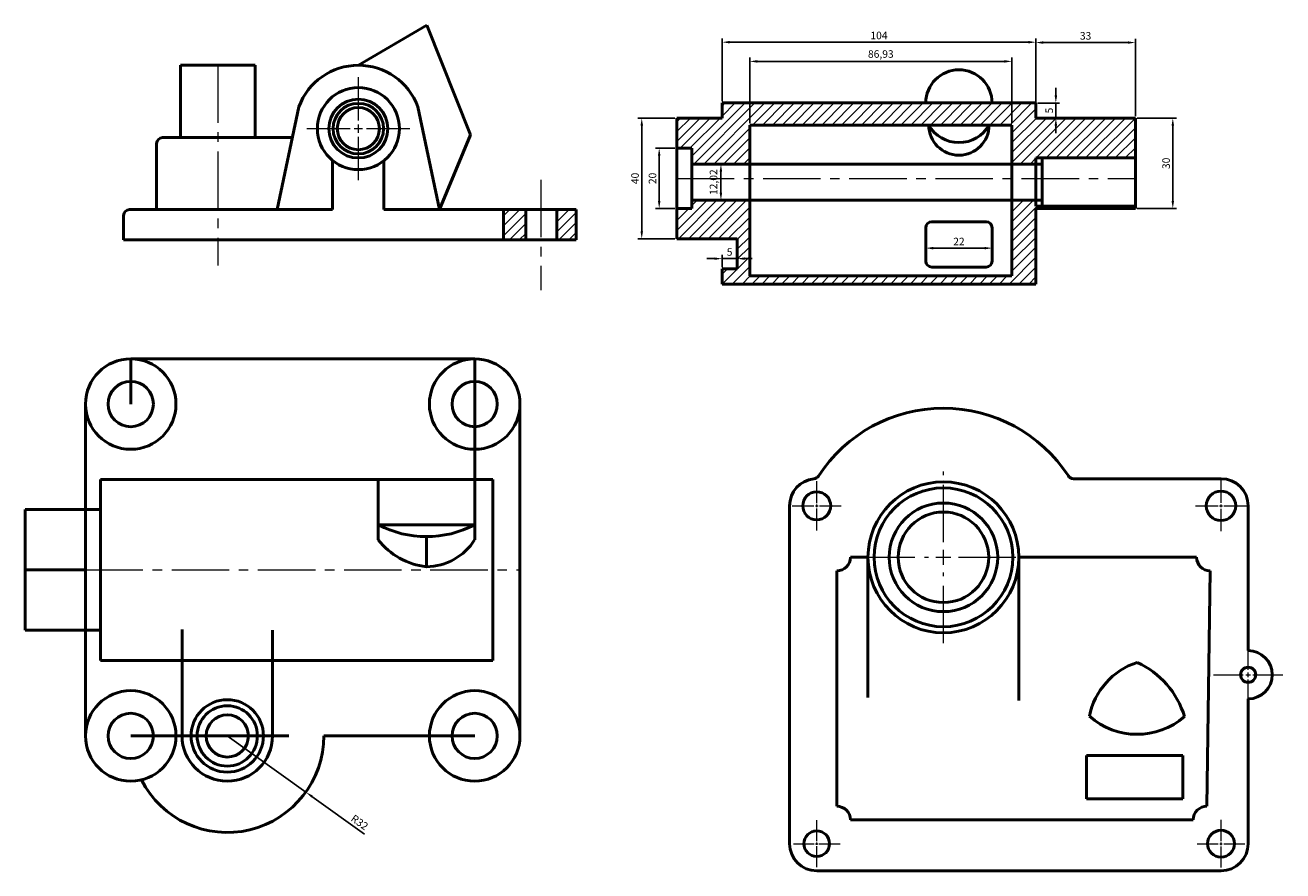
# Model space of a CAD drawing. Units: millimetres. Extents: x 1096 to 1848, y 1781 to 2075.
# Tile 1 of 2: x 1096 to 1513, y 1795 to 2075. Entities that reach past the tile are written whole.
import ezdxf

# ---------------------------------------------------------------- set-up
doc = ezdxf.new("R2010")
doc.units = ezdxf.units.MM
doc.linetypes.add('CENTER2', pattern=[28.575, 19.05, -3.175, 3.175, -3.175])
for name, color, linetype, lineweight in [('M-CNTR', 1, 'CENTER2', 18), ('M-DIMS', 2, 'Continuous', 25), ('M-HATC', 8, 'Continuous', 18), ('M-OUTL', 7, 'Continuous', 50)]:
    doc.layers.add(name, color=color, linetype=linetype, lineweight=lineweight)
doc.styles.get("Standard").update_dxf_attribs({"font": 'arial.ttf'})
doc.dimstyles.new('ISO-25', dxfattribs={"dimtxt": 2.5, "dimasz": 2.5, "dimexe": 1.25, "dimexo": 0.625, "dimtad": 1, "dimtxsty": 'Standard', "dimcen": 2.5, "dimadec": 0, "dimazin": 0, "dimtfac": 1, "dimtmove": 0, "dimatfit": 3, "dimfxl": 1, "dimarcsym": 0})

# ---------------------------------------------------------------- blocks, each defined once
blk = doc.blocks.new('*U1')
at = {"layer": 'M-CNTR', "color": 0, "transparency": 16777216}
for p, q in [((0, 2.72), (0, 17.09)), ((-17.09, 0), (-2.72, 0)), ((2.72, 0), (17.09, 0)), ((0, -17.09), (0, -2.72))]:
    blk.add_line(p, q, dxfattribs=at)
at = {"layer": 'M-CNTR', "color": 0, "linetype": 'Continuous', "transparency": 16777216}
for p, q in [((-1.36, 0), (1.36, 0)), ((0, -1.36), (0, 1.36))]:
    blk.add_line(p, q, dxfattribs=at)
blk = doc.blocks.new('*D2')
at = {"layer": 'Defpoints', "color": 0, "transparency": 16777216}
for p in [(1431.45, 2069.78), (1327.45, 2049.62), (1431.45, 2049.62)]:
    blk.add_point(p, dxfattribs=at)
at = {"layer": 'M-DIMS', "color": 0, "lineweight": -2, "transparency": 16777216}
for p, q in [((1327.45, 2050.25), (1327.45, 2071.03)), ((1329.95, 2069.78), (1428.95, 2069.78)), ((1431.45, 2050.25), (1431.45, 2071.03))]:
    blk.add_line(p, q, dxfattribs=at)
at = {"layer": 'M-DIMS', "color": 0, "transparency": 16777216}
for points in [[(1329.95, 2070.2), (1329.95, 2069.37), (1327.45, 2069.78)], [(1428.95, 2070.2), (1428.95, 2069.37), (1431.45, 2069.78)]]:
    blk.add_solid(points, dxfattribs=at)
at = {"layer": 'M-DIMS', "color": 0, "transparency": 16777216, "insert": (1379.45, 2071.68), "char_height": 2.5, "attachment_point": 5}
blk.add_mtext('104', dxfattribs=at)
blk = doc.blocks.new('*D3')
at = {"layer": 'Defpoints', "color": 0, "transparency": 16777216}
for p in [(1423.53, 2063.42), (1336.6, 2042.31), (1423.53, 2042.31)]:
    blk.add_point(p, dxfattribs=at)
at = {"layer": 'M-DIMS', "color": 0, "lineweight": -2, "transparency": 16777216}
for p, q in [((1336.6, 2042.94), (1336.6, 2064.67)), ((1423.53, 2042.94), (1423.53, 2064.67)), ((1339.1, 2063.42), (1421.03, 2063.42))]:
    blk.add_line(p, q, dxfattribs=at)
at = {"layer": 'M-DIMS', "color": 0, "transparency": 16777216}
for points in [[(1339.1, 2063.83), (1339.1, 2063), (1336.6, 2063.42)], [(1421.03, 2063.83), (1421.03, 2063), (1423.53, 2063.42)]]:
    blk.add_solid(points, dxfattribs=at)
at = {"layer": 'M-DIMS', "color": 0, "transparency": 16777216, "insert": (1380.07, 2065.54), "char_height": 2.5, "attachment_point": 5}
blk.add_mtext('86,93', dxfattribs=at)
blk = doc.blocks.new('*D4')
at = {"layer": 'Defpoints', "color": 0, "transparency": 16777216}
for p in [(1464.45, 2044.62), (1464.45, 2014.62), (1476.86, 2014.62)]:
    blk.add_point(p, dxfattribs=at)
at = {"layer": 'M-DIMS', "color": 0, "lineweight": -2, "transparency": 16777216}
for p, q in [((1465.08, 2044.62), (1478.11, 2044.62)), ((1476.86, 2042.12), (1476.86, 2017.12)), ((1465.08, 2014.62), (1478.11, 2014.62))]:
    blk.add_line(p, q, dxfattribs=at)
at = {"layer": 'M-DIMS', "color": 0, "transparency": 16777216}
for points in [[(1476.44, 2042.12), (1477.27, 2042.12), (1476.86, 2044.62)], [(1476.44, 2017.12), (1477.27, 2017.12), (1476.86, 2014.62)]]:
    blk.add_solid(points, dxfattribs=at)
at = {"layer": 'M-DIMS', "color": 0, "transparency": 16777216, "insert": (1474.96, 2029.62), "char_height": 2.5, "attachment_point": 5, "rotation": 90}
blk.add_mtext('30', dxfattribs=at)
blk = doc.blocks.new('*D5')
at = {"layer": 'Defpoints', "color": 0, "transparency": 16777216}
for p in [(1394.96, 2002.73), (1416.96, 2002.73), (1416.96, 2001.51)]:
    blk.add_point(p, dxfattribs=at)
at = {"layer": 'M-DIMS', "color": 0, "lineweight": -2, "transparency": 16777216}
for p, q in [((1394.96, 2002.11), (1394.96, 2000.26)), ((1397.46, 2001.51), (1414.46, 2001.51)), ((1416.96, 2002.11), (1416.96, 2000.26))]:
    blk.add_line(p, q, dxfattribs=at)
at = {"layer": 'M-DIMS', "color": 0, "transparency": 16777216}
for points in [[(1397.46, 2001.92), (1397.46, 2001.09), (1394.96, 2001.51)], [(1414.46, 2001.92), (1414.46, 2001.09), (1416.96, 2001.51)]]:
    blk.add_solid(points, dxfattribs=at)
at = {"layer": 'M-DIMS', "color": 0, "transparency": 16777216, "insert": (1405.96, 2003.39), "char_height": 2.5, "attachment_point": 5}
blk.add_mtext('22', dxfattribs=at)
blk = doc.blocks.new('*D6')
at = {"layer": 'Defpoints', "color": 0, "transparency": 16777216}
for p in [(1332.45, 1998.03), (1327.45, 1994.62), (1332.45, 1994.62)]:
    blk.add_point(p, dxfattribs=at)
at = {"layer": 'M-DIMS', "color": 0, "lineweight": -2, "transparency": 16777216}
for p, q in [((1324.95, 1998.03), (1322.45, 1998.03)), ((1327.45, 1995.25), (1327.45, 1999.28)), ((1327.45, 1998.03), (1332.45, 1998.03)), ((1332.45, 1995.25), (1332.45, 1999.28)), ((1334.95, 1998.03), (1337.45, 1998.03))]:
    blk.add_line(p, q, dxfattribs=at)
at = {"layer": 'M-DIMS', "color": 0, "transparency": 16777216}
for points in [[(1324.95, 1998.44), (1324.95, 1997.61), (1327.45, 1998.03)], [(1334.95, 1998.44), (1334.95, 1997.61), (1332.45, 1998.03)]]:
    blk.add_solid(points, dxfattribs=at)
at = {"layer": 'M-DIMS', "color": 0, "transparency": 16777216, "insert": (1329.95, 1999.92), "char_height": 2.5, "attachment_point": 5}
blk.add_mtext('5', dxfattribs=at)
blk = doc.blocks.new('*D7')
at = {"layer": 'Defpoints', "color": 0, "transparency": 16777216}
for p in [(1312.45, 2044.62), (1300.83, 2004.62), (1312.45, 2004.62)]:
    blk.add_point(p, dxfattribs=at)
at = {"layer": 'M-DIMS', "color": 0, "lineweight": -2, "transparency": 16777216}
for p, q in [((1311.83, 2044.62), (1299.58, 2044.62)), ((1300.83, 2042.12), (1300.83, 2007.12)), ((1311.83, 2004.62), (1299.58, 2004.62))]:
    blk.add_line(p, q, dxfattribs=at)
at = {"layer": 'M-DIMS', "color": 0, "transparency": 16777216}
for points in [[(1300.41, 2042.12), (1301.25, 2042.12), (1300.83, 2044.62)], [(1300.41, 2007.12), (1301.25, 2007.12), (1300.83, 2004.62)]]:
    blk.add_solid(points, dxfattribs=at)
at = {"layer": 'M-DIMS', "color": 0, "transparency": 16777216, "insert": (1298.93, 2024.62), "char_height": 2.5, "attachment_point": 5, "rotation": 90}
blk.add_mtext('40', dxfattribs=at)
blk = doc.blocks.new('*D8')
at = {"layer": 'Defpoints', "color": 0, "transparency": 16777216}
for p in [(1312.45, 2034.62), (1306.61, 2014.62), (1312.45, 2014.62)]:
    blk.add_point(p, dxfattribs=at)
at = {"layer": 'M-DIMS', "color": 0, "lineweight": -2, "transparency": 16777216}
for p, q in [((1311.83, 2034.62), (1305.36, 2034.62)), ((1306.61, 2032.12), (1306.61, 2017.12)), ((1311.83, 2014.62), (1305.36, 2014.62))]:
    blk.add_line(p, q, dxfattribs=at)
at = {"layer": 'M-DIMS', "color": 0, "transparency": 16777216}
for points in [[(1306.19, 2032.12), (1307.03, 2032.12), (1306.61, 2034.62)], [(1306.19, 2017.12), (1307.03, 2017.12), (1306.61, 2014.62)]]:
    blk.add_solid(points, dxfattribs=at)
at = {"layer": 'M-DIMS', "color": 0, "transparency": 16777216, "insert": (1304.71, 2024.62), "char_height": 2.5, "attachment_point": 5, "rotation": 90}
blk.add_mtext('20', dxfattribs=at)
blk = doc.blocks.new('*D9')
at = {"layer": 'Defpoints', "color": 0, "transparency": 16777216}
for p in [(1317.45, 2029.39), (1317.45, 2017.37), (1327.07, 2017.37)]:
    blk.add_point(p, dxfattribs=at)
at = {"layer": 'M-DIMS', "color": 0, "lineweight": -2, "transparency": 16777216}
for p, q in [((1318.08, 2029.39), (1328.32, 2029.39)), ((1327.07, 2026.89), (1327.07, 2019.87)), ((1318.08, 2017.37), (1328.32, 2017.37))]:
    blk.add_line(p, q, dxfattribs=at)
at = {"layer": 'M-DIMS', "color": 0, "transparency": 16777216}
for points in [[(1326.65, 2026.89), (1327.48, 2026.89), (1327.07, 2029.39)], [(1326.65, 2019.87), (1327.48, 2019.87), (1327.07, 2017.37)]]:
    blk.add_solid(points, dxfattribs=at)
at = {"layer": 'M-DIMS', "color": 0, "transparency": 16777216, "insert": (1324.94, 2023.38), "char_height": 2.5, "attachment_point": 5, "rotation": 90}
blk.add_mtext('12,02', dxfattribs=at)
blk = doc.blocks.new('*D10')
at = {"layer": 'Defpoints', "color": 0, "transparency": 16777216}
for p in [(1464.45, 2069.66), (1431.45, 2044.62), (1464.45, 2044.62)]:
    blk.add_point(p, dxfattribs=at)
at = {"layer": 'M-DIMS', "color": 0, "lineweight": -2, "transparency": 16777216}
for p, q in [((1431.45, 2045.25), (1431.45, 2070.91)), ((1433.95, 2069.66), (1461.95, 2069.66)), ((1464.45, 2045.25), (1464.45, 2070.91))]:
    blk.add_line(p, q, dxfattribs=at)
at = {"layer": 'M-DIMS', "color": 0, "transparency": 16777216}
for points in [[(1433.95, 2070.08), (1433.95, 2069.24), (1431.45, 2069.66)], [(1461.95, 2070.08), (1461.95, 2069.24), (1464.45, 2069.66)]]:
    blk.add_solid(points, dxfattribs=at)
at = {"layer": 'M-DIMS', "color": 0, "transparency": 16777216, "insert": (1447.95, 2071.56), "char_height": 2.5, "attachment_point": 5}
blk.add_mtext('33', dxfattribs=at)
blk = doc.blocks.new('*D11')
at = {"layer": 'Defpoints', "color": 0, "transparency": 16777216}
for p in [(1431.45, 2049.62), (1431.45, 2044.62), (1438.09, 2044.62)]:
    blk.add_point(p, dxfattribs=at)
at = {"layer": 'M-DIMS', "color": 0, "lineweight": -2, "transparency": 16777216}
for p, q in [((1438.09, 2052.12), (1438.09, 2054.62)), ((1432.08, 2049.62), (1439.34, 2049.62)), ((1438.09, 2049.62), (1438.09, 2044.62)), ((1432.08, 2044.62), (1439.34, 2044.62)), ((1438.09, 2042.12), (1438.09, 2039.62))]:
    blk.add_line(p, q, dxfattribs=at)
at = {"layer": 'M-DIMS', "color": 0, "transparency": 16777216}
for points in [[(1437.68, 2052.12), (1438.51, 2052.12), (1438.09, 2049.62)], [(1437.68, 2042.12), (1438.51, 2042.12), (1438.09, 2044.62)]]:
    blk.add_solid(points, dxfattribs=at)
at = {"layer": 'M-DIMS', "color": 0, "transparency": 16777216, "insert": (1436.2, 2047.12), "char_height": 2.5, "attachment_point": 5, "rotation": 90}
blk.add_mtext('5', dxfattribs=at)
blk = doc.blocks.new('*D12')
at = {"layer": 'Defpoints', "color": 0, "transparency": 16777216}
for p in [(1163.45, 1839.83), (1189.47, 1821.21)]:
    blk.add_point(p, dxfattribs=at)
at = {"layer": 'M-DIMS', "color": 0, "lineweight": -2, "transparency": 16777216}
for p, q in [((1163.45, 1839.83), (1189.47, 1821.21)), ((1208.96, 1807.28), (1191.51, 1819.76))]:
    blk.add_line(p, q, dxfattribs=at)
at = {"layer": 'M-DIMS', "color": 0, "transparency": 16777216}
blk.add_solid([(1191.75, 1820.1), (1191.27, 1819.42), (1189.47, 1821.21)], dxfattribs=at)
at = {"layer": 'M-DIMS', "color": 0, "transparency": 16777216, "insert": (1207.13, 1810.92), "char_height": 2.5, "attachment_point": 5, "rotation": 324.4294}
blk.add_mtext('R32', dxfattribs=at)
blk = doc.blocks.new('*U29')
at = {"layer": 'M-CNTR', "color": 0, "transparency": 16777216}
for p, q in [((0, 1.6), (0, 11.5)), ((-11.5, 0), (-1.6, 0)), ((1.6, 0), (11.5, 0)), ((0, -11.5), (0, -1.6))]:
    blk.add_line(p, q, dxfattribs=at)
at = {"layer": 'M-CNTR', "color": 0, "linetype": 'Continuous', "transparency": 16777216}
for p, q in [((-0.8, 0), (0.8, 0)), ((0, -0.8), (0, 0.8))]:
    blk.add_line(p, q, dxfattribs=at)
blk = doc.blocks.new('*U30')
at = {"layer": 'M-CNTR', "color": 0, "transparency": 16777216}
for p, q in [((0, 0.98), (0, 8.4)), ((-8.4, 0), (-0.98, 0)), ((0.98, 0), (8.4, 0)), ((0, -8.4), (0, -0.98))]:
    blk.add_line(p, q, dxfattribs=at)
at = {"layer": 'M-CNTR', "color": 0, "linetype": 'Continuous', "transparency": 16777216}
for p, q in [((-0.49, 0), (0.49, 0)), ((0, -0.49), (0, 0.49))]:
    blk.add_line(p, q, dxfattribs=at)
blk = doc.blocks.new('*U31')
at = {"layer": 'M-CNTR', "color": 0, "transparency": 16777216}
for p, q in [((0, 0.93), (0, 8.14)), ((-8.14, 0), (-0.93, 0)), ((0.93, 0), (8.14, 0)), ((0, -8.14), (0, -0.93))]:
    blk.add_line(p, q, dxfattribs=at)
at = {"layer": 'M-CNTR', "color": 0, "linetype": 'Continuous', "transparency": 16777216}
for p, q in [((-0.46, 0), (0.46, 0)), ((0, -0.46), (0, 0.46))]:
    blk.add_line(p, q, dxfattribs=at)
blk = doc.blocks.new('*U32')
at = {"layer": 'M-CNTR', "color": 0, "transparency": 16777216}
for p, q in [((0, 0.85), (0, 7.75)), ((-7.75, 0), (-0.85, 0)), ((0.85, 0), (7.75, 0)), ((0, -7.75), (0, -0.85))]:
    blk.add_line(p, q, dxfattribs=at)
at = {"layer": 'M-CNTR', "color": 0, "linetype": 'Continuous', "transparency": 16777216}
for p, q in [((-0.42, 0), (0.42, 0)), ((0, -0.42), (0, 0.42))]:
    blk.add_line(p, q, dxfattribs=at)
blk = doc.blocks.new('*U33')
at = {"layer": 'M-CNTR', "color": 0, "transparency": 16777216}
for p, q in [((0, 0.89), (0, 7.94)), ((-7.94, 0), (-0.89, 0)), ((0.89, 0), (7.94, 0)), ((0, -7.94), (0, -0.89))]:
    blk.add_line(p, q, dxfattribs=at)
at = {"layer": 'M-CNTR', "color": 0, "linetype": 'Continuous', "transparency": 16777216}
for p, q in [((-0.44, 0), (0.44, 0)), ((0, -0.44), (0, 0.44))]:
    blk.add_line(p, q, dxfattribs=at)
blk = doc.blocks.new('*U34')
at = {"layer": 'M-CNTR', "color": 0, "transparency": 16777216}
for p, q in [((0, 5), (0, 28.5)), ((-28.5, 0), (-5, 0)), ((5, 0), (28.5, 0)), ((0, -28.5), (0, -5))]:
    blk.add_line(p, q, dxfattribs=at)
at = {"layer": 'M-CNTR', "color": 0, "linetype": 'Continuous', "transparency": 16777216}
for p, q in [((-2.5, 0), (2.5, 0)), ((0, -2.5), (0, 2.5))]:
    blk.add_line(p, q, dxfattribs=at)

msp = doc.modelspace()

# ---------------------------------------------------------------- hatches: boundary and pattern name
at = {"layer": 'M-HATC'}
h = msp.add_hatch(dxfattribs=at)
h.set_pattern_fill('ANSI31', color=256, scale=0.73)
h.paths.add_polyline_path([(1336.601, 2042.315), (1423.534, 2042.315), (1423.534, 2029.393), (1431.451, 2029.393), (1431.451, 2031.393), (1464.451, 2031.393), (1464.451, 2044.624), (1431.451, 2044.624), (1431.451, 2049.624), (1327.451, 2049.624), (1327.451, 2044.624), (1312.451, 2044.624), (1312.451, 2034.624), (1317.451, 2034.624), (1317.451, 2029.393), (1336.601, 2029.393)])
h.paths.add_polyline_path([(1336.601, 2017.37), (1317.451, 2017.37), (1317.451, 2014.624), (1312.451, 2014.624), (1312.451, 2004.624), (1332.451, 2004.624), (1332.451, 1994.624), (1327.451, 1994.624), (1327.451, 1989.624), (1405.964, 1989.624), (1405.964, 1992.315), (1336.601, 1992.315)])
h.paths.add_polyline_path([(1431.451, 2009.624), (1431.451, 2014.624), (1464.451, 2014.624), (1464.451, 2015.37), (1431.451, 2015.37), (1431.451, 2017.37), (1423.534, 2017.37), (1423.534, 1992.315), (1405.964, 1992.315), (1405.964, 1989.624), (1431.451, 1989.624)])
h = msp.add_hatch(dxfattribs=at)
h.set_pattern_fill('ANSI31', color=256, scale=0.73)
h.paths.add_polyline_path([(1262.355, 2014.293), (1255.005, 2014.293), (1255.005, 2004.293), (1262.355, 2004.293)])
h.paths.add_polyline_path([(1279.065, 2014.293), (1272.699, 2014.293), (1272.699, 2004.293), (1279.065, 2004.293)])

# ---------------------------------------------------------------- linework, layer by layer
at = {"layer": 'M-CNTR'}
for p, q in [((1160.311, 2062.13), (1160.311, 1995.777)), ((1267.391, 2024.177), (1267.391, 1987.597)), ((1312.451, 2024.624), (1464.451, 2024.606)), ((1116.445, 1894.829), (1260.445, 1894.829))]:
    msp.add_line(p, q, dxfattribs=at)
at = {"layer": 'M-OUTL'}
for p, q in [((1229.589, 2075.428), (1206.891, 2062.13)), ((1244.098, 2039.119), (1229.589, 2075.428)), ((1172.715, 2062.13), (1147.906, 2062.13)), ((1147.906, 2038.156), (1147.906, 2062.13)), ((1172.715, 2062.13), (1172.715, 2038.156)), ((1187.159, 2048.317), (1179.988, 2014.293)), ((1226.623, 2048.317), (1233.794, 2014.293)), ((1327.451, 2049.624), (1431.451, 2049.624)), ((1327.451, 2049.624), (1327.451, 2044.624)), ((1427.964, 2049.624), (1405.964, 2049.624)), ((1431.451, 2049.624), (1431.451, 2044.624)), ((1327.451, 2044.624), (1312.451, 2044.624)), ((1312.451, 2004.624), (1312.451, 2044.624)), ((1312.451, 2044.624), (1312.451, 2034.624)), ((1431.451, 2044.624), (1464.451, 2044.624)), ((1464.451, 2044.624), (1464.451, 2014.624)), ((1233.794, 2014.293), (1244.098, 2039.119)), ((1336.601, 2042.315), (1423.534, 2042.315)), ((1336.601, 2042.315), (1336.601, 1992.315)), ((1423.534, 2042.315), (1423.534, 1992.315)), ((1140.018, 2036.156), (1140.018, 2014.293)), ((1185.018, 2038.156), (1142.018, 2038.156)), ((1312.451, 2034.624), (1317.451, 2034.624)), ((1317.451, 2034.624), (1317.451, 2014.624)), ((1198.366, 2030.546), (1198.366, 2014.293)), ((1215.347, 2014.293), (1215.347, 2030.491)), ((1431.451, 2029.393), (1431.451, 2031.393)), ((1431.451, 2031.393), (1464.451, 2031.393)), ((1433.599, 2031.393), (1433.599, 2015.37)), ((1317.451, 2029.393), (1336.601, 2029.393)), ((1336.601, 2029.393), (1433.599, 2029.393)), ((1431.451, 2017.37), (1431.451, 2029.393)), ((1131.065, 2014.293), (1174.065, 2014.293)), ((1165.74, 2014.293), (1198.366, 2014.293)), ((1174.065, 2014.293), (1173.065, 2014.293)), ((1198.366, 2014.293), (1174.065, 2014.293)), ((1215.347, 2014.293), (1245.065, 2014.293)), ((1215.347, 2014.293), (1260.548, 2014.293)), ((1279.065, 2014.293), (1245.065, 2014.293)), ((1255.005, 2014.293), (1255.005, 2004.293)), ((1262.355, 2004.293), (1262.355, 2014.293)), ((1272.699, 2014.293), (1272.699, 2004.293)), ((1279.065, 2004.293), (1279.065, 2014.293)), ((1317.451, 2014.624), (1312.451, 2014.624)), ((1336.601, 2017.37), (1317.451, 2017.37)), ((1336.601, 2017.37), (1433.599, 2017.37)), ((1431.451, 2017.37), (1431.451, 2015.37)), ((1431.451, 2015.37), (1464.451, 2015.37)), ((1464.451, 2014.624), (1431.451, 2014.624)), ((1431.451, 2014.624), (1431.451, 2009.624)), ((1129.065, 2004.293), (1129.065, 2012.293)), ((1405.964, 2010.232), (1396.964, 2010.232)), ((1414.964, 2010.232), (1405.964, 2010.232)), ((1431.451, 2009.624), (1431.451, 1989.624)), ((1394.964, 2008.232), (1394.964, 1997.232)), ((1416.964, 1997.232), (1416.964, 2008.232)), ((1139.065, 2004.293), (1129.065, 2004.293)), ((1209.065, 2004.293), (1139.065, 2004.293)), ((1209.065, 2004.293), (1279.065, 2004.293)), ((1332.451, 2004.624), (1312.451, 2004.624)), ((1332.451, 1994.624), (1332.451, 2004.624)), ((1327.451, 1989.624), (1327.451, 1994.624)), ((1327.451, 1994.624), (1332.451, 1994.624)), ((1396.964, 1995.232), (1414.964, 1995.232)), ((1431.451, 1989.624), (1327.451, 1989.624)), ((1423.534, 1992.315), (1336.601, 1992.315)), ((1131.445, 1964.829), (1245.445, 1964.829)), ((1131.445, 1964.829), (1131.445, 1949.829)), ((1245.445, 1964.829), (1245.445, 1949.829)), ((1116.445, 1949.829), (1116.445, 1839.829)), ((1245.445, 1949.829), (1245.445, 1909.829)), ((1260.445, 1949.829), (1260.445, 1839.829)), ((1121.445, 1914.829), (1121.445, 1924.829)), ((1121.445, 1924.829), (1251.445, 1924.829)), ((1213.445, 1909.829), (1213.445, 1924.829)), ((1251.445, 1864.829), (1251.445, 1924.829)), ((1492.831, 1925.095), (1443.909, 1925.095)), ((1096.445, 1894.829), (1096.445, 1914.829)), ((1096.445, 1914.829), (1121.445, 1914.829)), ((1121.445, 1914.829), (1121.445, 1874.829)), ((1349.831, 1916.095), (1349.831, 1804.095)), ((1501.831, 1868.095), (1501.831, 1916.095)), ((1245.445, 1909.829), (1213.445, 1909.829)), ((1213.445, 1909.829), (1213.445, 1904.829)), ((1245.445, 1909.829), (1245.445, 1904.829)), ((1229.445, 1905.873), (1229.445, 1895.873)), ((1375.821, 1899.026), (1370.016, 1899.026)), ((1375.821, 1899.026), (1375.821, 1852.587)), ((1425.821, 1899.026), (1484.754, 1899.026)), ((1425.821, 1899.026), (1425.821, 1851.572)), ((1116.445, 1894.829), (1096.445, 1894.829)), ((1096.445, 1874.829), (1096.445, 1894.829)), ((1365.516, 1894.526), (1365.516, 1816.492)), ((1488.178, 1816.492), (1489.195, 1894.526)), ((1121.445, 1874.829), (1096.445, 1874.829)), ((1121.445, 1874.829), (1121.445, 1864.829)), ((1148.445, 1839.829), (1148.445, 1875.066)), ((1178.445, 1839.829), (1178.445, 1874.886)), ((1121.445, 1864.829), (1251.445, 1864.829)), ((1501.831, 1804.095), (1501.831, 1852.095)), ((1131.445, 1839.829), (1163.445, 1839.829)), ((1163.445, 1839.829), (1183.858, 1839.829)), ((1195.445, 1839.829), (1245.445, 1839.829)), ((1480.214, 1833.301), (1448.249, 1833.301)), ((1448.249, 1833.301), (1448.249, 1818.957)), ((1480.214, 1818.957), (1480.214, 1833.301)), ((1448.249, 1818.957), (1458.543, 1818.957)), ((1458.543, 1818.957), (1480.214, 1818.957)), ((1370.016, 1811.992), (1483.619, 1811.992)), ((1358.831, 1795.095), (1492.831, 1795.095))]:
    msp.add_line(p, q, dxfattribs=at)
for centre, radius in [((1206.891, 2041.13), 13.59), ((1206.891, 2041.13), 9.738), ((1206.891, 2041.13), 8.382), ((1206.891, 2041.13), 6.983), ((1131.445, 1949.829), 15), ((1245.445, 1949.829), 15), ((1131.445, 1949.829), 7.5), ((1245.445, 1949.829), 7.5), ((1400.821, 1899.026), 25), ((1400.821, 1899.026), 23), ((1358.831, 1916.095), 4.637), ((1492.831, 1916.095), 4.897), ((1400.821, 1899.026), 18), ((1400.821, 1899.026), 15), ((1501.831, 1860.095), 2.5), ((1131.445, 1839.829), 15), ((1163.445, 1839.829), 12), ((1245.445, 1839.829), 15), ((1131.445, 1839.829), 7.5), ((1163.445, 1839.829), 10), ((1163.445, 1839.829), 7), ((1245.445, 1839.829), 7.5), ((1358.831, 1804.095), 4.245), ((1492.831, 1804.095), 4.438)]:
    msp.add_circle(centre, radius, dxfattribs=at)
for centre, radius, start, end in [((1206.891, 2041.13), 21, 20.01347, 159.98653), ((1405.964, 2049.624), 11, 0, 180), ((1405.964, 2042.315), 10, 180, 360), ((1405.964, 2047.971), 11.489, 209.49263, 330.50737), ((1142.018, 2036.156), 2, 90, 180), ((1131.065, 2012.293), 2, 90, 180), ((1396.964, 2008.232), 2, 90, 180), ((1414.964, 2008.232), 2, 0, 90), ((1396.964, 1997.232), 2, 180, 270), ((1414.964, 1997.232), 2, 270, 0), ((1400.821, 1899.026), 49.424, 33.08143, 146.99679), ((1358.831, 1916.095), 9, 95.92946, 180), ((1357.694, 1927.036), 2, 275.92946, 326.99679), ((1443.909, 1927.095), 2, 213.08143, 270), ((1492.831, 1916.095), 9, 0, 90), ((1229.445, 1940.205), 34.333, 242.22318, 297.77682), ((1232.364, 1919.856), 24.161, 218.46111, 263.06215), ((1229.137, 1915.193), 19.322, 270.91302, 327.56373), ((1365.516, 1899.026), 4.5, 270, 0), ((1489.254, 1899.026), 4.5, 180, 269.25333), ((1501.831, 1860.095), 8, 270, 90), ((1472.304, 1841.834), 23.498, 107.98188, 168.92904), ((1453.104, 1837.918), 28.856, 16.76032, 65.54481), ((1465.05, 1864.185), 23.834, 228.45546, 311.15256), ((1163.445, 1839.829), 32, 207.10957, 0), ((1163.445, 1839.829), 15, 180, 0), ((1365.516, 1811.992), 4.5, 0, 90), ((1488.119, 1811.992), 4.5, 89.25333, 180), ((1358.831, 1804.095), 9, 180, 270), ((1492.831, 1804.095), 9, 270, 0)]:
    msp.add_arc(centre, radius, start, end, dxfattribs=at)

# ---------------------------------------------------------------- block references
at = {"layer": 'M-CNTR'}
for name, p in [('*U1', (1206.891, 2041.13)), ('*U34', (1400.821, 1899.026)), ('*U31', (1358.831, 1916.095)), ('*U30', (1492.831, 1916.095)), ('*U29', (1501.831, 1860.095)), ('*U32', (1358.831, 1804.095)), ('*U33', (1492.831, 1804.095))]:
    msp.add_blockref(name, p, dxfattribs=at)

# ---------------------------------------------------------------- dimensions: what is measured, and where the dimension line sits
at = {"layer": 'M-DIMS'}
for base, p1, p2, picture, middle in [((1431.451, 2069.782), (1327.451, 2049.624), (1431.451, 2049.624), '*D2', (1379.451, 2071.684)), ((1464.451, 2069.661), (1431.451, 2044.624), (1464.451, 2044.624), '*D10', (1447.951, 2071.563)), ((1423.534, 2063.416), (1336.601, 2042.315), (1423.534, 2042.315), '*D3', (1380.068, 2065.543)), ((1332.451, 1998.028), (1327.451, 1994.624), (1332.451, 1994.624), '*D6', (1329.951, 1999.924)), ((1416.964, 2001.507), (1394.964, 2002.732), (1416.964, 2002.732), '*D5', (1405.964, 2003.387))]:
    dim = msp.add_linear_dim(base=base, p1=p1, p2=p2, dimstyle='ISO-25', override={"dimclrd": 0, "dimclre": 0, "dimclrt": 0}, dxfattribs=at)
    dim.commit()
    dim.dimension.update_dxf_attribs({"geometry": picture, "text_midpoint": middle})
for base, p1, p2, picture, middle in [((1438.094, 2044.624), (1431.451, 2049.624), (1431.451, 2044.624), '*D11', (1436.198, 2047.124)), ((1300.831, 2004.624), (1312.451, 2044.624), (1312.451, 2004.624), '*D7', (1298.93, 2024.624)), ((1476.858, 2014.624), (1464.451, 2044.624), (1464.451, 2014.624), '*D4', (1474.955, 2029.624)), ((1306.61, 2014.624), (1312.451, 2034.624), (1312.451, 2014.624), '*D8', (1304.708, 2024.624)), ((1327.068, 2017.37), (1317.451, 2029.393), (1317.451, 2017.37), '*D9', (1324.941, 2023.381))]:
    dim = msp.add_linear_dim(base=base, p1=p1, p2=p2, angle=90, dimstyle='ISO-25', override={"dimclrd": 0, "dimclre": 0, "dimclrt": 0}, dxfattribs=at)
    dim.commit()
    dim.dimension.update_dxf_attribs({"geometry": picture, "text_midpoint": middle})
dim = msp.add_radius_dim(center=(1163.445, 1839.829), mpoint=(1189.474, 1821.214), dimstyle='ISO-25', override={"dimclrd": 0, "dimclre": 0, "dimclrt": 0}, dxfattribs=at)
dim.commit()
dim.dimension.update_dxf_attribs({"geometry": '*D12', "text_midpoint": (1206.028, 1809.376), "dimtype": 164})

doc.saveas('drawing.dxf')
